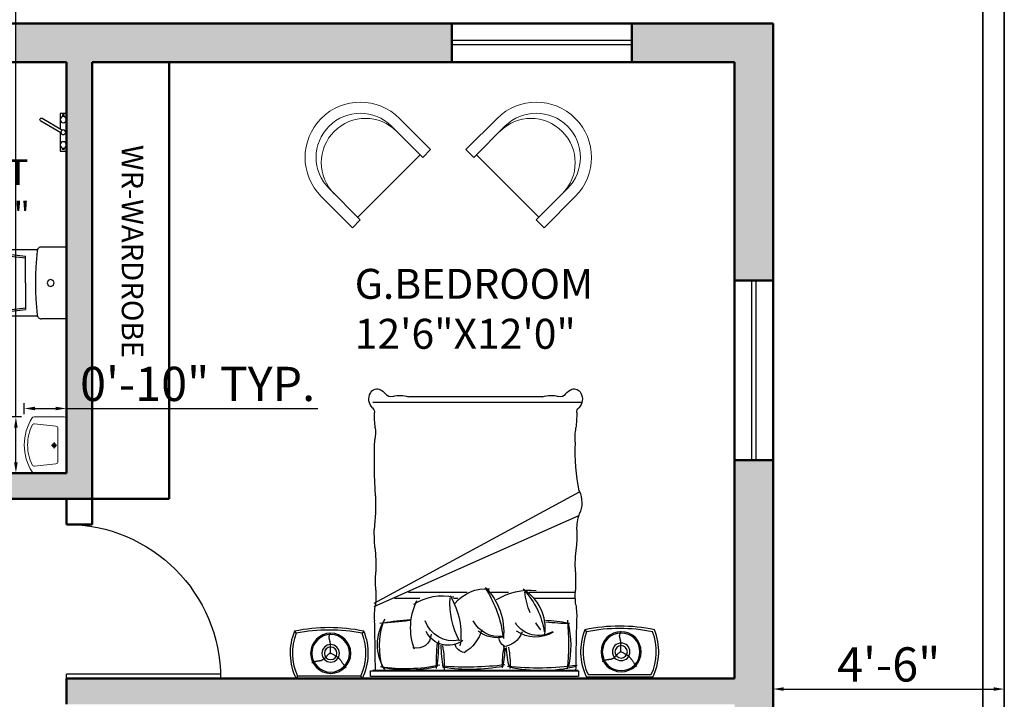
# Model space of a CAD drawing. Units: inches. Extents: x 3008 to 4088, y 1255 to 2137.
# Tile 29 of 30: x 3853 to 4083, y 1792 to 1951. Entities that reach past the tile are written whole.
import ezdxf

# ---------------------------------------------------------------- set-up
doc = ezdxf.new("R2010")
doc.units = ezdxf.units.IN
for name, color, linetype, lineweight in [('A-ANNO-DIMS', 2, 'Continuous', 18), ('A-ANNO-TEXT', 7, 'Continuous', 18), ('A-AREA-IDEN', 7, 'Continuous', 18), ('A-DOOR', 4, 'Continuous', 25), ('A-FLOR-FIXT', 8, 'Continuous', 18), ('A-FURN', 8, 'Continuous', 18), ('A-GLAZ', 4, 'Continuous', 25), ('A-WALL', 7, 'Continuous', 50), ('A-WALL-PATT', 8, 'Continuous', 13), ('C-PROP', 1, 'Continuous', 35)]:
    doc.layers.add(name, color=color, linetype=linetype, lineweight=lineweight)
doc.layers.add('SANTEH', color=7, linetype='Continuous')
doc.layers.add('TEFRİŞ', color=11, linetype='Continuous')
doc.styles.get("Standard").update_dxf_attribs({"font": 'arial.ttf'})
doc.dimstyles.new('ISO-25', dxfattribs={"dimtxt": 8, "dimasz": 2.5, "dimexe": 1.25, "dimexo": 0.625, "dimtad": 1, "dimdec": 1, "dimlunit": 3, "dimtxsty": 'Standard', "dimcen": 2.5, "dimadec": 0, "dimazin": 0, "dimtfac": 1, "dimtdec": 1, "dimtmove": 0, "dimatfit": 3, "dimfxl": 1, "dimarcsym": 0})

# ---------------------------------------------------------------- blocks, each defined once
blk = doc.blocks.new('*D34')
at = {"layer": 'A-ANNO-DIMS', "color": 0, "lineweight": -2, "transparency": 16777216}
for p, q in [((4028.94, 1793.63), (4028.94, 1793.01)), ((4031.44, 1794.26), (4080.44, 1794.26)), ((4082.94, 1793.63), (4082.94, 1793.01))]:
    blk.add_line(p, q, dxfattribs=at)
at = {"layer": 'A-ANNO-DIMS', "color": 0, "transparency": 16777216}
for points in [[(4031.44, 1794.68), (4031.44, 1793.84), (4028.94, 1794.26)], [(4080.44, 1794.68), (4080.44, 1793.84), (4082.94, 1794.26)]]:
    blk.add_solid(points, dxfattribs=at)
at = {"layer": 'Defpoints', "color": 0, "transparency": 16777216}
for p in [(4028.94, 1794.26), (4082.94, 1794.26), (4082.94, 1794.26)]:
    blk.add_point(p, dxfattribs=at)
at = {"layer": 'A-ANNO-DIMS', "color": 0, "transparency": 16777216, "insert": (4055.94, 1798.97), "char_height": 8, "attachment_point": 5}
blk.add_mtext('4\'-6"', dxfattribs=at)
blk = doc.blocks.new('WC 2 Symb_109')
at = {"layer": 'SANTEH'}
for p, q in [((0, 0), (0, 380)), ((0, 380), (132.4, 380)), ((153.6, 364.9), (506.8, 364.9)), ((506.3, 364.9), (215.7, 330.9)), ((506.3, 356), (215.7, 322)), ((215.7, 190), (215.7, 330.9)), ((215.7, 190), (215.7, 49.1)), ((506.3, 24), (215.7, 58)), ((153.8, 15.1), (506.8, 15.1)), ((506.3, 15.1), (215.7, 49.1)), ((0, 0), (132.4, 0))]:
    blk.add_line(p, q, dxfattribs=at)
for points in [[(154.6, 360.1), (153.9, 364.1), (152.3, 367.9), (150.2, 371.3), (147.4, 374.3), (144.1, 376.7), (140.5, 378.5), (136.5, 379.6), (132.4, 380)], [(506.8, 15.1), (569.2, 28.4), (622.2, 66.3), (657.6, 123.1), (670, 190), (657.6, 256.9), (622.2, 313.7), (569.2, 351.6), (506.8, 364.9)], [(154.6, 19.7), (158.6, 62.1), (161.4, 104.7), (163.1, 147.3), (163.7, 189.9), (163.1, 232.5), (161.4, 275.1), (158.6, 317.7), (154.6, 360.1)], [(506.3, 24), (565.5, 36.6), (615.7, 72.6), (649.2, 126.5), (661, 190), (649.2, 253.5), (615.7, 307.4), (565.5, 343.4), (506.3, 356)], [(132.4, 0), (136.5, 0.4), (140.4, 1.5), (144.1, 3.2), (147.3, 5.6), (150.1, 8.6), (152.3, 12), (153.8, 15.7), (154.6, 19.7)]]:
    blk.add_lwpolyline(points, dxfattribs=at)
blk.add_lwpolyline([(83.6, 208.5), (70.4, 203.1), (64.9, 190), (70.4, 176.9), (83.6, 171.5), (96.8, 176.9), (102.2, 190), (96.8, 203.1)], close=True, dxfattribs=at)
blk = doc.blocks.new('Faucet - kit sink top')
at = {"layer": 'SANTEH'}
for p, q in [((-5.5, -0.75), (-5.5, -1.25)), ((-4.94278, -0.75), (-5.5, -0.75)), ((-5.5, -1.25), (-4.94278, -1.25)), ((-0.14775, -1.7441), (3.56698, -8.1782)), ((4.43301, -7.6782), (0.71828, -1.2441)), ((4.94278, -0.75), (5.5, -0.75)), ((5.5, -1.25), (4.94278, -1.25)), ((5.5, -0.75), (5.5, -1.25))]:
    blk.add_line(p, q, dxfattribs=at)
blk.add_lwpolyline([(-0.00587, -2), (-6, -2), (-6, 0), (6, 0), (6, -2), (1.15195, -2)], dxfattribs=at)
for centre, radius in [((-4, -1), 1), ((4, -1), 1), ((0, -1), 0.75)]:
    blk.add_circle(centre, radius, dxfattribs=at)
blk.add_arc((4, -7.9282), 0.5, 210, 30, dxfattribs=at)
blk = doc.blocks.new('A$C2EBB240D')
for p, q in [((0, 355.8), (0, 86.6)), ((480, 375.8), (20, 375.8)), ((500, 355.8), (500, 86.6)), ((60.8, 89.8), (82.3, 282.2)), ((250, 300), (102.1, 300)), ((250, 300), (397.9, 300)), ((439.2, 89.8), (417.7, 282.2))]:
    blk.add_line(p, q)
for points in [[(275.2, 266.4), (219.4, 266.4)], [(247.3, 238.5), (247.3, 288.9)]]:
    blk.add_lwpolyline(points)
for centre, radius, start, end in [((20, 355.8), 20, 90, 180), ((480, 355.8), 20, 0, 90), ((102.1, 280), 20, 90, 173.64284), ((247.3, 266.4), 16.7, 90, 270), ((247.3, 266.4), 10, 90, 270), ((247.3, 266.4), 16.7, 270, 90), ((247.3, 266.4), 10, 270, 90), ((397.9, 280), 20, 6.35716, 90), ((80.7, 87.6), 20, 173.64284, 244.97956), ((419.3, 87.6), 20, 295.02044, 6.35716), ((20, 86.6), 20, 180, 237.68921), ((250, 450.3), 450.3, 237.68921, 270), ((250, 450.3), 420.3, 244.97956, 270), ((250, 450.3), 450.3, 270, 302.31079), ((250, 450.3), 420.3, 270, 295.02044), ((480, 86.6), 20, 302.31079, 0)]:
    blk.add_arc(centre, radius, start, end)
blk = doc.blocks.new('D1')
for p, q in [((1805.96, 1500.36), (1805.96, 1464.36)), ((1806.96, 1500.36), (1806.96, 1464.36)), ((1805.96, 1464.36), (1806.96, 1464.36))]:
    blk.add_line(p, q)
blk.add_arc((1805.96, 1464.36), 36, 0, 90)
blk = doc.blocks.new('12PSTG07')
at = {"color": 0, "linetype": 'ByBlock'}
for p, q in [((0, 15), (-12, 15)), ((0, 12), (0, 15)), ((-12, 12), (0, 12)), ((-1, -12), (-1, 12)), ((-12, -12), (0, -12)), ((0, -12), (0, -15)), ((0, -15), (-12, -15))]:
    blk.add_line(p, q, dxfattribs=at)
for centre, radius in [((-12, 0), 15), ((-12, 0), 12), ((-10, 0), 12)]:
    blk.add_arc(centre, radius, 90, 270, dxfattribs=at)
blk = doc.blocks.new('BED')
at = {"layer": 'TEFRİŞ'}
for p, q in [((2114.88, 1835.66), (2129.12, 1835.66)), ((2115.2, 1835.15), (2128.8, 1835.15)), ((2130.81, 1834.34), (2130.81, 1835.55)), ((2175.56, 1834.34), (2130.81, 1834.34)), ((2130.91, 1835.55), (2175.56, 1835.55)), ((2175, 1834.19), (2130.91, 1834.19)), ((2175.56, 1835.55), (2175.56, 1834.34)), ((2177.29, 1835.98), (2177.61, 1835.47)), ((2177.29, 1835.98), (2191.52, 1835.98)), ((2177.61, 1835.47), (2191.2, 1835.47)), ((2191.2, 1835.47), (2191.52, 1835.98)), ((2118.49, 1833.2), (2118.34, 1833.38)), ((2118.49, 1833.2), (2118.34, 1833.38)), ((2118.63, 1833.03), (2118.49, 1833.2)), ((2118.63, 1833.03), (2118.49, 1833.2)), ((2118.75, 1832.88), (2118.63, 1833.03)), ((2118.75, 1832.88), (2118.63, 1833.03)), ((2118.86, 1832.74), (2118.75, 1832.88)), ((2118.86, 1832.74), (2118.75, 1832.88)), ((2118.95, 1832.61), (2118.86, 1832.74)), ((2118.95, 1832.61), (2118.86, 1832.74)), ((2119.04, 1832.48), (2118.95, 1832.61)), ((2119.04, 1832.48), (2118.95, 1832.61)), ((2119.12, 1832.37), (2119.04, 1832.48)), ((2119.12, 1832.37), (2119.04, 1832.48)), ((2119.19, 1832.26), (2119.12, 1832.37)), ((2119.19, 1832.26), (2119.12, 1832.37)), ((2119.26, 1832.16), (2119.19, 1832.26)), ((2119.26, 1832.16), (2119.19, 1832.26)), ((2119.32, 1832.06), (2119.26, 1832.16)), ((2119.32, 1832.06), (2119.26, 1832.16)), ((2119.39, 1831.97), (2119.32, 1832.06)), ((2119.39, 1831.97), (2119.32, 1832.06)), ((2124.79, 1831.99), (2124.87, 1832.01)), ((2124.79, 1831.99), (2124.87, 1832.01)), ((2124.87, 1832.01), (2124.96, 1832.03)), ((2124.87, 1832.01), (2124.96, 1832.03)), ((2124.96, 1832.03), (2125.05, 1832.05)), ((2124.96, 1832.03), (2125.05, 1832.05)), ((2125.05, 1832.05), (2125.14, 1832.08)), ((2125.05, 1832.05), (2125.14, 1832.08)), ((2125.14, 1832.08), (2125.23, 1832.11)), ((2125.14, 1832.08), (2125.23, 1832.11)), ((2125.23, 1832.11), (2125.33, 1832.14)), ((2125.23, 1832.11), (2125.33, 1832.14)), ((2125.33, 1832.14), (2125.42, 1832.17)), ((2125.33, 1832.14), (2125.42, 1832.17)), ((2125.42, 1832.17), (2125.52, 1832.21)), ((2125.42, 1832.17), (2125.52, 1832.21)), ((2125.52, 1832.21), (2125.6, 1832.25)), ((2125.52, 1832.21), (2125.6, 1832.25)), ((2125.6, 1832.25), (2125.68, 1832.3)), ((2125.6, 1832.25), (2125.68, 1832.3)), ((2125.68, 1832.3), (2125.75, 1832.35)), ((2125.68, 1832.3), (2125.75, 1832.35)), ((2180.9, 1833.52), (2180.75, 1833.7)), ((2180.9, 1833.52), (2180.75, 1833.7)), ((2181.04, 1833.35), (2180.9, 1833.52)), ((2181.04, 1833.35), (2180.9, 1833.52)), ((2181.16, 1833.2), (2181.04, 1833.35)), ((2181.16, 1833.2), (2181.04, 1833.35)), ((2181.26, 1833.06), (2181.16, 1833.2)), ((2181.26, 1833.06), (2181.16, 1833.2)), ((2181.36, 1832.93), (2181.26, 1833.06)), ((2181.36, 1832.93), (2181.26, 1833.06)), ((2181.44, 1832.8), (2181.36, 1832.93)), ((2181.44, 1832.8), (2181.36, 1832.93)), ((2181.52, 1832.69), (2181.44, 1832.8)), ((2181.52, 1832.69), (2181.44, 1832.8)), ((2181.59, 1832.58), (2181.52, 1832.69)), ((2181.59, 1832.58), (2181.52, 1832.69)), ((2181.66, 1832.48), (2181.59, 1832.58)), ((2181.66, 1832.48), (2181.59, 1832.58)), ((2181.73, 1832.38), (2181.66, 1832.48)), ((2181.73, 1832.38), (2181.66, 1832.48)), ((2181.79, 1832.29), (2181.73, 1832.38)), ((2181.79, 1832.29), (2181.73, 1832.38)), ((2181.85, 1832.21), (2181.79, 1832.29)), ((2181.85, 1832.21), (2181.79, 1832.29)), ((2181.92, 1832.13), (2181.85, 1832.21)), ((2181.92, 1832.13), (2181.85, 1832.21)), ((2181.97, 1832.05), (2181.92, 1832.13)), ((2181.97, 1832.05), (2181.92, 1832.13)), ((2182.03, 1831.97), (2181.97, 1832.05)), ((2182.03, 1831.97), (2181.97, 1832.05)), ((2185.82, 1831.99), (2185.89, 1832.03)), ((2185.82, 1831.99), (2185.89, 1832.03)), ((2185.89, 1832.03), (2185.96, 1832.06)), ((2185.89, 1832.03), (2185.96, 1832.06)), ((2185.96, 1832.06), (2186.03, 1832.09)), ((2185.96, 1832.06), (2186.03, 1832.09)), ((2186.03, 1832.09), (2186.1, 1832.12)), ((2186.03, 1832.09), (2186.1, 1832.12)), ((2186.1, 1832.12), (2186.17, 1832.14)), ((2186.1, 1832.12), (2186.17, 1832.14)), ((2186.17, 1832.14), (2186.24, 1832.16)), ((2186.17, 1832.14), (2186.24, 1832.16)), ((2186.24, 1832.16), (2186.32, 1832.18)), ((2186.24, 1832.16), (2186.32, 1832.18)), ((2186.32, 1832.18), (2186.39, 1832.19)), ((2186.32, 1832.18), (2186.39, 1832.19)), ((2186.39, 1832.19), (2186.46, 1832.21)), ((2186.39, 1832.19), (2186.46, 1832.21)), ((2186.46, 1832.21), (2186.53, 1832.22)), ((2186.46, 1832.21), (2186.53, 1832.22)), ((2186.53, 1832.22), (2186.61, 1832.23)), ((2186.53, 1832.22), (2186.61, 1832.23)), ((2186.61, 1832.23), (2186.68, 1832.23)), ((2186.61, 1832.23), (2186.68, 1832.23)), ((2186.68, 1832.23), (2186.75, 1832.24)), ((2186.68, 1832.23), (2186.75, 1832.24)), ((2186.75, 1832.24), (2186.82, 1832.25)), ((2186.75, 1832.24), (2186.82, 1832.25)), ((2186.82, 1832.25), (2186.9, 1832.26)), ((2186.82, 1832.25), (2186.9, 1832.26)), ((2186.9, 1832.26), (2186.97, 1832.27)), ((2186.9, 1832.26), (2186.97, 1832.27)), ((2186.97, 1832.27), (2187.04, 1832.28)), ((2186.97, 1832.27), (2187.04, 1832.28)), ((2187.04, 1832.28), (2187.12, 1832.3)), ((2187.04, 1832.28), (2187.12, 1832.3)), ((2187.12, 1832.3), (2187.2, 1832.31)), ((2187.12, 1832.3), (2187.2, 1832.31)), ((2187.2, 1832.31), (2187.28, 1832.33)), ((2187.2, 1832.31), (2187.28, 1832.33)), ((2187.28, 1832.33), (2187.36, 1832.35)), ((2187.28, 1832.33), (2187.36, 1832.35)), ((2187.36, 1832.35), (2187.45, 1832.37)), ((2187.36, 1832.35), (2187.45, 1832.37)), ((2187.45, 1832.37), (2187.54, 1832.4)), ((2187.45, 1832.37), (2187.54, 1832.4)), ((2187.54, 1832.4), (2187.64, 1832.43)), ((2187.54, 1832.4), (2187.64, 1832.43)), ((2187.64, 1832.43), (2187.74, 1832.46)), ((2187.64, 1832.43), (2187.74, 1832.46)), ((2187.74, 1832.46), (2187.83, 1832.49)), ((2187.74, 1832.46), (2187.83, 1832.49)), ((2187.83, 1832.49), (2187.92, 1832.53)), ((2187.83, 1832.49), (2187.92, 1832.53)), ((2187.92, 1832.53), (2188.01, 1832.57)), ((2187.92, 1832.53), (2188.01, 1832.57)), ((2188.01, 1832.57), (2188.09, 1832.62)), ((2188.01, 1832.57), (2188.09, 1832.62)), ((2188.09, 1832.62), (2188.15, 1832.67)), ((2188.09, 1832.62), (2188.15, 1832.67)), ((2119.45, 1831.89), (2119.39, 1831.97)), ((2119.45, 1831.89), (2119.39, 1831.97)), ((2119.51, 1831.81), (2119.45, 1831.89)), ((2119.51, 1831.81), (2119.45, 1831.89)), ((2119.57, 1831.73), (2119.51, 1831.81)), ((2119.57, 1831.73), (2119.51, 1831.81)), ((2119.63, 1831.65), (2119.57, 1831.73)), ((2119.63, 1831.65), (2119.57, 1831.73)), ((2119.69, 1831.58), (2119.63, 1831.65)), ((2119.69, 1831.58), (2119.63, 1831.65)), ((2119.75, 1831.51), (2119.69, 1831.58)), ((2119.75, 1831.51), (2119.69, 1831.58)), ((2119.81, 1831.44), (2119.75, 1831.51)), ((2119.81, 1831.44), (2119.75, 1831.51)), ((2119.87, 1831.38), (2119.81, 1831.44)), ((2119.87, 1831.38), (2119.81, 1831.44)), ((2119.93, 1831.31), (2119.87, 1831.38)), ((2119.93, 1831.31), (2119.87, 1831.38)), ((2119.99, 1831.25), (2119.93, 1831.31)), ((2119.99, 1831.25), (2119.93, 1831.31)), ((2120.05, 1831.2), (2119.99, 1831.25)), ((2120.05, 1831.2), (2119.99, 1831.25)), ((2120.12, 1831.14), (2120.05, 1831.2)), ((2120.12, 1831.14), (2120.05, 1831.2)), ((2120.18, 1831.09), (2120.12, 1831.14)), ((2120.18, 1831.09), (2120.12, 1831.14)), ((2120.25, 1831.04), (2120.18, 1831.09)), ((2120.25, 1831.04), (2120.18, 1831.09)), ((2120.32, 1830.99), (2120.25, 1831.04)), ((2120.32, 1830.99), (2120.25, 1831.04)), ((2120.39, 1830.94), (2120.32, 1830.99)), ((2120.39, 1830.94), (2120.32, 1830.99)), ((2120.47, 1830.9), (2120.39, 1830.94)), ((2120.47, 1830.9), (2120.39, 1830.94)), ((2120.54, 1830.85), (2120.47, 1830.9)), ((2120.54, 1830.85), (2120.47, 1830.9)), ((2120.62, 1830.8), (2120.54, 1830.85)), ((2120.62, 1830.8), (2120.54, 1830.85)), ((2120.7, 1830.75), (2120.62, 1830.8)), ((2120.7, 1830.75), (2120.62, 1830.8)), ((2120.79, 1830.7), (2120.7, 1830.75)), ((2120.79, 1830.7), (2120.7, 1830.75)), ((2120.88, 1830.65), (2120.79, 1830.7)), ((2120.88, 1830.65), (2120.79, 1830.7)), ((2120.98, 1830.59), (2120.88, 1830.65)), ((2120.98, 1830.59), (2120.88, 1830.65)), ((2121.09, 1830.52), (2120.98, 1830.59)), ((2121.09, 1830.52), (2120.98, 1830.59)), ((2121.21, 1830.45), (2121.09, 1830.52)), ((2121.21, 1830.45), (2121.09, 1830.52)), ((2121.34, 1830.38), (2121.21, 1830.45)), ((2121.34, 1830.38), (2121.21, 1830.45)), ((2121.49, 1830.29), (2121.34, 1830.38)), ((2121.49, 1830.29), (2121.34, 1830.38)), ((2121.66, 1830.21), (2121.49, 1830.29)), ((2121.66, 1830.21), (2121.49, 1830.29)), ((2121.66, 1830.18), (2121.87, 1830.29)), ((2121.66, 1830.18), (2121.87, 1830.29)), ((2121.85, 1830.11), (2121.66, 1830.21)), ((2121.85, 1830.11), (2121.66, 1830.21)), ((2121.74, 1829.99), (2121.73, 1829.83)), ((2121.74, 1829.99), (2121.73, 1829.83)), ((2121.76, 1830.38), (2121.74, 1830.17)), ((2121.76, 1830.38), (2121.74, 1830.17)), ((2121.74, 1830.17), (2121.74, 1829.99)), ((2121.74, 1830.17), (2121.74, 1829.99)), ((2121.87, 1830.29), (2122.04, 1830.4)), ((2121.87, 1830.29), (2122.04, 1830.4)), ((2122.04, 1830.4), (2122.2, 1830.51)), ((2122.04, 1830.4), (2122.2, 1830.51)), ((2122.2, 1830.51), (2122.33, 1830.61)), ((2122.2, 1830.51), (2122.33, 1830.61)), ((2122.33, 1830.61), (2122.45, 1830.72)), ((2122.33, 1830.61), (2122.45, 1830.72)), ((2122.45, 1830.72), (2122.55, 1830.82)), ((2122.45, 1830.72), (2122.55, 1830.82)), ((2122.55, 1830.82), (2122.64, 1830.91)), ((2122.55, 1830.82), (2122.64, 1830.91)), ((2122.64, 1830.91), (2122.72, 1831.01)), ((2122.64, 1830.91), (2122.72, 1831.01)), ((2122.72, 1831.01), (2122.8, 1831.09)), ((2122.72, 1831.01), (2122.8, 1831.09)), ((2122.8, 1831.09), (2122.87, 1831.18)), ((2122.8, 1831.09), (2122.87, 1831.18)), ((2122.87, 1831.18), (2122.94, 1831.26)), ((2122.87, 1831.18), (2122.94, 1831.26)), ((2122.94, 1831.26), (2123.01, 1831.33)), ((2122.94, 1831.26), (2123.01, 1831.33)), ((2123.01, 1831.33), (2123.08, 1831.4)), ((2123.01, 1831.33), (2123.08, 1831.4)), ((2123.08, 1831.4), (2123.14, 1831.46)), ((2123.08, 1831.4), (2123.14, 1831.46)), ((2123.14, 1831.46), (2123.21, 1831.52)), ((2123.14, 1831.46), (2123.21, 1831.52)), ((2123.21, 1831.52), (2123.27, 1831.58)), ((2123.21, 1831.52), (2123.27, 1831.58)), ((2123.27, 1831.58), (2123.34, 1831.63)), ((2123.27, 1831.58), (2123.34, 1831.63)), ((2123.34, 1831.63), (2123.41, 1831.67)), ((2123.34, 1831.63), (2123.41, 1831.67)), ((2123.41, 1831.67), (2123.48, 1831.71)), ((2123.41, 1831.67), (2123.48, 1831.71)), ((2123.48, 1831.71), (2123.55, 1831.74)), ((2123.48, 1831.71), (2123.55, 1831.74)), ((2123.55, 1831.74), (2123.62, 1831.77)), ((2123.55, 1831.74), (2123.62, 1831.77)), ((2123.62, 1831.77), (2123.69, 1831.8)), ((2123.62, 1831.77), (2123.69, 1831.8)), ((2123.69, 1831.8), (2123.77, 1831.82)), ((2123.69, 1831.8), (2123.77, 1831.82)), ((2123.77, 1831.82), (2123.84, 1831.84)), ((2123.77, 1831.82), (2123.84, 1831.84)), ((2123.84, 1831.84), (2123.91, 1831.86)), ((2123.84, 1831.84), (2123.91, 1831.86)), ((2123.91, 1831.86), (2123.98, 1831.87)), ((2123.91, 1831.86), (2123.98, 1831.87)), ((2123.98, 1831.87), (2124.06, 1831.89)), ((2123.98, 1831.87), (2124.06, 1831.89)), ((2124.06, 1831.89), (2124.13, 1831.9)), ((2124.06, 1831.89), (2124.13, 1831.9)), ((2124.13, 1831.9), (2124.2, 1831.91)), ((2124.13, 1831.9), (2124.2, 1831.91)), ((2124.2, 1831.91), (2124.27, 1831.91)), ((2124.2, 1831.91), (2124.27, 1831.91)), ((2124.27, 1831.91), (2124.35, 1831.92)), ((2124.27, 1831.91), (2124.35, 1831.92)), ((2124.35, 1831.92), (2124.42, 1831.93)), ((2124.35, 1831.92), (2124.42, 1831.93)), ((2124.42, 1831.93), (2124.49, 1831.94)), ((2124.42, 1831.93), (2124.49, 1831.94)), ((2124.49, 1831.94), (2124.56, 1831.95)), ((2124.49, 1831.94), (2124.56, 1831.95)), ((2124.56, 1831.95), (2124.64, 1831.96)), ((2124.56, 1831.95), (2124.64, 1831.96)), ((2124.64, 1831.96), (2124.71, 1831.98)), ((2124.64, 1831.96), (2124.71, 1831.98)), ((2124.71, 1831.98), (2124.79, 1831.99)), ((2124.71, 1831.98), (2124.79, 1831.99)), ((2182.09, 1831.9), (2182.03, 1831.97)), ((2182.09, 1831.9), (2182.03, 1831.97)), ((2182.15, 1831.83), (2182.09, 1831.9)), ((2182.15, 1831.83), (2182.09, 1831.9)), ((2182.21, 1831.76), (2182.15, 1831.83)), ((2182.21, 1831.76), (2182.15, 1831.83)), ((2182.27, 1831.7), (2182.21, 1831.76)), ((2182.27, 1831.7), (2182.21, 1831.76)), ((2182.33, 1831.63), (2182.27, 1831.7)), ((2182.33, 1831.63), (2182.27, 1831.7)), ((2182.4, 1831.57), (2182.33, 1831.63)), ((2182.4, 1831.57), (2182.33, 1831.63)), ((2182.46, 1831.52), (2182.4, 1831.57)), ((2182.46, 1831.52), (2182.4, 1831.57)), ((2182.52, 1831.46), (2182.46, 1831.52)), ((2182.52, 1831.46), (2182.46, 1831.52)), ((2182.59, 1831.41), (2182.52, 1831.46)), ((2182.59, 1831.41), (2182.52, 1831.46)), ((2182.66, 1831.36), (2182.59, 1831.41)), ((2182.66, 1831.36), (2182.59, 1831.41)), ((2182.73, 1831.31), (2182.66, 1831.36)), ((2182.73, 1831.31), (2182.66, 1831.36)), ((2182.8, 1831.26), (2182.73, 1831.31)), ((2182.8, 1831.26), (2182.73, 1831.31)), ((2182.87, 1831.22), (2182.8, 1831.26)), ((2182.87, 1831.22), (2182.8, 1831.26)), ((2182.95, 1831.17), (2182.87, 1831.22)), ((2182.95, 1831.17), (2182.87, 1831.22)), ((2183.03, 1831.12), (2182.95, 1831.17)), ((2183.03, 1831.12), (2182.95, 1831.17)), ((2183.11, 1831.07), (2183.03, 1831.12)), ((2183.11, 1831.07), (2183.03, 1831.12)), ((2183.2, 1831.02), (2183.11, 1831.07)), ((2183.2, 1831.02), (2183.11, 1831.07)), ((2183.29, 1830.97), (2183.2, 1831.02)), ((2183.29, 1830.97), (2183.2, 1831.02)), ((2183.39, 1830.91), (2183.29, 1830.97)), ((2183.39, 1830.91), (2183.29, 1830.97)), ((2183.49, 1830.84), (2183.39, 1830.91)), ((2183.49, 1830.84), (2183.39, 1830.91)), ((2183.61, 1830.77), (2183.49, 1830.84)), ((2183.61, 1830.77), (2183.49, 1830.84)), ((2183.75, 1830.7), (2183.61, 1830.77)), ((2183.75, 1830.7), (2183.61, 1830.77)), ((2183.9, 1830.61), (2183.75, 1830.7)), ((2183.9, 1830.61), (2183.75, 1830.7)), ((2184.06, 1830.53), (2183.9, 1830.61)), ((2184.06, 1830.53), (2183.9, 1830.61)), ((2184.25, 1830.43), (2184.06, 1830.53)), ((2184.25, 1830.43), (2184.06, 1830.53)), ((2184.07, 1830.5), (2184.27, 1830.61)), ((2184.07, 1830.5), (2184.27, 1830.61)), ((2184.15, 1830.49), (2184.14, 1830.31)), ((2184.15, 1830.49), (2184.14, 1830.31)), ((2184.14, 1830.31), (2184.14, 1830.15)), ((2184.14, 1830.31), (2184.14, 1830.15)), ((2184.14, 1830.15), (2184.14, 1830.01)), ((2184.14, 1830.15), (2184.14, 1830.01)), ((2184.14, 1830.01), (2184.14, 1829.89)), ((2184.14, 1830.01), (2184.14, 1829.89)), ((2184.14, 1829.89), (2184.14, 1829.77)), ((2184.14, 1829.89), (2184.14, 1829.77)), ((2184.17, 1830.7), (2184.15, 1830.49)), ((2184.17, 1830.7), (2184.15, 1830.49)), ((2184.27, 1830.61), (2184.45, 1830.72)), ((2184.27, 1830.61), (2184.45, 1830.72)), ((2184.45, 1830.72), (2184.6, 1830.83)), ((2184.45, 1830.72), (2184.6, 1830.83)), ((2184.6, 1830.83), (2184.74, 1830.93)), ((2184.6, 1830.83), (2184.74, 1830.93)), ((2184.74, 1830.93), (2184.85, 1831.04)), ((2184.74, 1830.93), (2184.85, 1831.04)), ((2184.85, 1831.04), (2184.95, 1831.14)), ((2184.85, 1831.04), (2184.95, 1831.14)), ((2184.95, 1831.14), (2185.05, 1831.23)), ((2184.95, 1831.14), (2185.05, 1831.23)), ((2185.05, 1831.23), (2185.13, 1831.33)), ((2185.05, 1831.23), (2185.13, 1831.33)), ((2185.13, 1831.33), (2185.21, 1831.41)), ((2185.13, 1831.33), (2185.21, 1831.41)), ((2185.21, 1831.41), (2185.28, 1831.5)), ((2185.21, 1831.41), (2185.28, 1831.5)), ((2185.28, 1831.5), (2185.35, 1831.58)), ((2185.28, 1831.5), (2185.35, 1831.58)), ((2185.35, 1831.58), (2185.42, 1831.65)), ((2185.35, 1831.58), (2185.42, 1831.65)), ((2185.42, 1831.65), (2185.48, 1831.72)), ((2185.42, 1831.65), (2185.48, 1831.72)), ((2185.48, 1831.72), (2185.55, 1831.78)), ((2185.48, 1831.72), (2185.55, 1831.78)), ((2185.55, 1831.78), (2185.61, 1831.84)), ((2185.55, 1831.78), (2185.61, 1831.84)), ((2185.61, 1831.84), (2185.68, 1831.9)), ((2185.61, 1831.84), (2185.68, 1831.9)), ((2185.68, 1831.9), (2185.75, 1831.95)), ((2185.68, 1831.9), (2185.75, 1831.95)), ((2185.75, 1831.95), (2185.82, 1831.99)), ((2185.75, 1831.95), (2185.82, 1831.99)), ((2121.73, 1829.83), (2121.73, 1829.69)), ((2121.73, 1829.83), (2121.73, 1829.69)), ((2121.73, 1829.69), (2121.73, 1829.57)), ((2121.73, 1829.69), (2121.73, 1829.57)), ((2121.73, 1829.57), (2121.73, 1829.45)), ((2121.73, 1829.57), (2121.73, 1829.45)), ((2121.73, 1829.45), (2121.74, 1829.35)), ((2121.73, 1829.45), (2121.74, 1829.35)), ((2121.74, 1828.89), (2121.73, 1828.8)), ((2121.74, 1828.89), (2121.73, 1828.8)), ((2121.73, 1828.8), (2121.73, 1828.72)), ((2121.73, 1828.8), (2121.73, 1828.72)), ((2121.73, 1828.72), (2121.73, 1828.64)), ((2121.73, 1828.72), (2121.73, 1828.64)), ((2121.73, 1828.64), (2121.73, 1828.56)), ((2121.73, 1828.64), (2121.73, 1828.56)), ((2121.73, 1828.56), (2121.73, 1828.48)), ((2121.73, 1828.56), (2121.73, 1828.48)), ((2121.73, 1828.48), (2121.73, 1828.4)), ((2121.73, 1828.48), (2121.73, 1828.4)), ((2121.73, 1828.4), (2121.73, 1828.33)), ((2121.73, 1828.4), (2121.73, 1828.33)), ((2121.73, 1828.33), (2121.74, 1828.25)), ((2121.73, 1828.33), (2121.74, 1828.25)), ((2121.74, 1829.35), (2121.74, 1829.25)), ((2121.74, 1829.35), (2121.74, 1829.25)), ((2121.74, 1829.25), (2121.74, 1829.16)), ((2121.74, 1829.25), (2121.74, 1829.16)), ((2121.74, 1829.16), (2121.74, 1829.06)), ((2121.74, 1829.16), (2121.74, 1829.06)), ((2121.74, 1829.06), (2121.74, 1828.97)), ((2121.74, 1829.06), (2121.74, 1828.97)), ((2121.74, 1828.97), (2121.74, 1828.89)), ((2121.74, 1828.97), (2121.74, 1828.89)), ((2121.74, 1828.25), (2121.75, 1828.18)), ((2121.74, 1828.25), (2121.75, 1828.18)), ((2121.75, 1828.18), (2121.75, 1828.1)), ((2121.75, 1828.18), (2121.75, 1828.1)), ((2121.75, 1828.1), (2121.76, 1828.03)), ((2121.75, 1828.1), (2121.76, 1828.03)), ((2121.76, 1828.03), (2121.78, 1827.95)), ((2121.76, 1828.03), (2121.78, 1827.95)), ((2121.78, 1827.95), (2121.79, 1827.88)), ((2121.78, 1827.95), (2121.79, 1827.88)), ((2121.79, 1827.88), (2121.8, 1827.8)), ((2121.79, 1827.88), (2121.8, 1827.8)), ((2121.8, 1827.8), (2121.82, 1827.72)), ((2121.8, 1827.8), (2121.82, 1827.72)), ((2184.14, 1829.04), (2184.13, 1828.96)), ((2184.14, 1829.04), (2184.13, 1828.96)), ((2184.13, 1828.96), (2184.13, 1828.88)), ((2184.13, 1828.96), (2184.13, 1828.88)), ((2184.13, 1828.88), (2184.13, 1828.8)), ((2184.13, 1828.88), (2184.13, 1828.8)), ((2184.13, 1828.8), (2184.14, 1828.72)), ((2184.13, 1828.8), (2184.14, 1828.72)), ((2184.14, 1829.77), (2184.14, 1829.67)), ((2184.14, 1829.77), (2184.14, 1829.67)), ((2184.14, 1829.67), (2184.15, 1829.57)), ((2184.14, 1829.67), (2184.15, 1829.57)), ((2184.15, 1829.38), (2184.14, 1829.29)), ((2184.15, 1829.38), (2184.14, 1829.29)), ((2184.14, 1829.29), (2184.14, 1829.21)), ((2184.14, 1829.29), (2184.14, 1829.21)), ((2184.14, 1829.21), (2184.14, 1829.12)), ((2184.14, 1829.21), (2184.14, 1829.12)), ((2184.14, 1829.12), (2184.14, 1829.04)), ((2184.14, 1829.12), (2184.14, 1829.04)), ((2184.14, 1828.72), (2184.14, 1828.65)), ((2184.14, 1828.72), (2184.14, 1828.65)), ((2184.14, 1828.65), (2184.15, 1828.57)), ((2184.14, 1828.65), (2184.15, 1828.57)), ((2184.15, 1829.57), (2184.15, 1829.48)), ((2184.15, 1829.57), (2184.15, 1829.48)), ((2184.15, 1829.48), (2184.15, 1829.38)), ((2184.15, 1829.48), (2184.15, 1829.38)), ((2184.15, 1828.57), (2184.15, 1828.5)), ((2184.15, 1828.57), (2184.15, 1828.5)), ((2184.15, 1828.5), (2184.16, 1828.42)), ((2184.15, 1828.5), (2184.16, 1828.42)), ((2184.16, 1828.42), (2184.17, 1828.35)), ((2184.16, 1828.42), (2184.17, 1828.35)), ((2184.17, 1828.35), (2184.18, 1828.27)), ((2184.17, 1828.35), (2184.18, 1828.27)), ((2184.18, 1828.27), (2184.19, 1828.2)), ((2184.18, 1828.27), (2184.19, 1828.2)), ((2184.19, 1828.2), (2184.21, 1828.12)), ((2184.19, 1828.2), (2184.21, 1828.12)), ((2184.21, 1828.12), (2184.22, 1828.04)), ((2184.21, 1828.12), (2184.22, 1828.04)), ((2184.22, 1828.04), (2184.24, 1827.97)), ((2184.22, 1828.04), (2184.24, 1827.97)), ((2184.24, 1827.97), (2184.26, 1827.89)), ((2184.24, 1827.97), (2184.26, 1827.89)), ((2184.26, 1827.89), (2184.28, 1827.81)), ((2184.26, 1827.89), (2184.28, 1827.81)), ((2184.28, 1827.81), (2184.3, 1827.73)), ((2184.28, 1827.81), (2184.3, 1827.73)), ((2121.78, 1825.93), (2121.74, 1825.8)), ((2121.78, 1825.93), (2121.74, 1825.8)), ((2121.83, 1826.06), (2121.78, 1825.93)), ((2121.83, 1826.06), (2121.78, 1825.93)), ((2121.82, 1827.72), (2121.84, 1827.65)), ((2121.82, 1827.72), (2121.84, 1827.65)), ((2121.87, 1826.19), (2121.83, 1826.06)), ((2121.87, 1826.19), (2121.83, 1826.06)), ((2121.84, 1827.65), (2121.85, 1827.57)), ((2121.84, 1827.65), (2121.85, 1827.57)), ((2121.85, 1827.57), (2121.87, 1827.49)), ((2121.85, 1827.57), (2121.87, 1827.49)), ((2121.87, 1827.49), (2121.89, 1827.41)), ((2121.87, 1827.49), (2121.89, 1827.41)), ((2121.91, 1826.31), (2121.87, 1826.19)), ((2121.91, 1826.31), (2121.87, 1826.19)), ((2121.89, 1827.41), (2121.91, 1827.33)), ((2121.89, 1827.41), (2121.91, 1827.33)), ((2121.91, 1827.33), (2121.93, 1827.26)), ((2121.91, 1827.33), (2121.93, 1827.26)), ((2121.95, 1826.42), (2121.91, 1826.31)), ((2121.95, 1826.42), (2121.91, 1826.31)), ((2121.93, 1827.26), (2121.95, 1827.18)), ((2121.93, 1827.26), (2121.95, 1827.18)), ((2121.95, 1827.18), (2121.97, 1827.09)), ((2121.95, 1827.18), (2121.97, 1827.09)), ((2121.97, 1826.54), (2121.95, 1826.42)), ((2121.97, 1826.54), (2121.95, 1826.42)), ((2121.97, 1827.09), (2121.99, 1827.01)), ((2121.97, 1827.09), (2121.99, 1827.01)), ((2121.99, 1826.64), (2121.97, 1826.54)), ((2121.99, 1826.64), (2121.97, 1826.54)), ((2121.99, 1827.01), (2122, 1826.93)), ((2121.99, 1827.01), (2122, 1826.93)), ((2122, 1826.74), (2121.99, 1826.64)), ((2122, 1826.74), (2121.99, 1826.64)), ((2122, 1826.93), (2122.01, 1826.84)), ((2122, 1826.93), (2122.01, 1826.84)), ((2122.01, 1826.84), (2122, 1826.74)), ((2122.01, 1826.84), (2122, 1826.74)), ((2129.46, 1825.49), (2129.09, 1825.93)), ((2176.94, 1825.81), (2177.31, 1826.25)), ((2184.19, 1826.25), (2184.14, 1826.12)), ((2184.19, 1826.25), (2184.14, 1826.12)), ((2184.23, 1826.38), (2184.19, 1826.25)), ((2184.23, 1826.38), (2184.19, 1826.25)), ((2184.28, 1826.51), (2184.23, 1826.38)), ((2184.28, 1826.51), (2184.23, 1826.38)), ((2184.32, 1826.63), (2184.28, 1826.51)), ((2184.32, 1826.63), (2184.28, 1826.51)), ((2184.3, 1827.73), (2184.32, 1827.65)), ((2184.3, 1827.73), (2184.32, 1827.65)), ((2184.32, 1827.65), (2184.34, 1827.58)), ((2184.32, 1827.65), (2184.34, 1827.58)), ((2184.35, 1826.74), (2184.32, 1826.63)), ((2184.35, 1826.74), (2184.32, 1826.63)), ((2184.34, 1827.58), (2184.36, 1827.5)), ((2184.34, 1827.58), (2184.36, 1827.5)), ((2184.38, 1826.86), (2184.35, 1826.74)), ((2184.38, 1826.86), (2184.35, 1826.74)), ((2184.36, 1827.5), (2184.38, 1827.41)), ((2184.36, 1827.5), (2184.38, 1827.41)), ((2184.38, 1827.41), (2184.4, 1827.33)), ((2184.38, 1827.41), (2184.4, 1827.33)), ((2184.4, 1826.96), (2184.38, 1826.86)), ((2184.4, 1826.96), (2184.38, 1826.86)), ((2184.4, 1827.33), (2184.41, 1827.25)), ((2184.4, 1827.33), (2184.41, 1827.25)), ((2184.41, 1827.06), (2184.4, 1826.96)), ((2184.41, 1827.06), (2184.4, 1826.96)), ((2184.41, 1827.25), (2184.41, 1827.16)), ((2184.41, 1827.25), (2184.41, 1827.16)), ((2184.41, 1827.16), (2184.41, 1827.06)), ((2184.41, 1827.16), (2184.41, 1827.06)), ((2191.87, 1825.81), (2191.5, 1826.25)), ((2174.77, 1819.77), (2130.6, 1795.83)), ((2174.77, 1820.53), (2130.76, 1800.91)), ((2140.43, 1818.69), (2131.53, 1818.69)), ((2141.43, 1817.4), (2131.53, 1817.4)), ((2149.62, 1817.4), (2145.88, 1817.4)), ((2167.36, 1817.4), (2154.77, 1817.4)), ((2157.71, 1818.69), (2156.77, 1818.69)), ((2170.41, 1818.69), (2164.92, 1818.69)), ((2175, 1776.57), (2130.11, 1776.57)), ((2138.52, 1775.41), (2167.39, 1775.41))]:
    blk.add_line(p, q, dxfattribs=at)
for centre, radius, start, end in [((2126, 1830.19), 12.39, 153.8162, 202.314), ((2126, 1830.19), 11.88, 155.3335, 201.0157), ((2118, 1830.19), 11.88, 338.9843, 24.6665), ((2118, 1830.19), 12.39, 337.686, 26.1838), ((2188.4, 1830.51), 12.39, 153.8162, 202.314), ((2188.4, 1830.51), 11.88, 155.3335, 201.0157), ((2180.41, 1830.51), 11.88, 338.9843, 24.6665), ((2180.41, 1830.51), 12.39, 337.686, 26.1838), ((2122, 1861.35), 36.12, 258.6773, 281.3227), ((2184.41, 1861.67), 36.63, 258.2443, 281.7557), ((2184.41, 1861.67), 36.12, 258.6773, 281.3227), ((2122, 1861.35), 36.63, 258.2443, 281.7557)]:
    blk.add_arc(centre, radius, start, end, dxfattribs=at)
at = {"layer": 'TEFRİŞ', "extrusion": (0, 0, -1)}
for centre, major_axis, ratio, start_param, end_param in [((2121.68, 1830.24), (-3.05, -3.05), 1, 3.926991, 10.210176), ((2121.68, 1830.24), (2.86, -2.86), 1, 5.497787, 11.780972), ((2121.68, 1830.24), (2.86, -2.86), 1, 5.497787, 11.780972), ((2206.14, 1830.73), (-52.86, -52.86), 1, 0.767743, 0.83177), ((2138.85, 1803.05), (-22.1, 22.1), 1, 0.544604, 1.006234), ((2154.12, 1796.61), (-26.46, 26.46), 1, 0.596409, 0.940188), ((2168.35, 1789.27), (-1.33, 44.62), 0.875277, -0.163954, 0.163954), ((2167.6, 1797.72), (-0.51, 36.47), 0.865194, -0.185965, 0.185965), ((2184.09, 1830.56), (-3.05, -3.05), 1, 3.926991, 10.210176), ((2184.09, 1830.56), (2.86, -2.86), 1, 5.497787, 11.780972), ((2184.09, 1830.56), (2.86, -2.86), 1, 5.497787, 11.780972), ((2121.68, 1830.24), (1.33, -1.33), 1, 5.497787, 11.780972), ((2121.68, 1830.24), (1.33, -1.33), 1, 5.497787, 11.780972), ((2139.43, 1773.84), (-42.35, 42.35), 1, 0.646251, 0.896949), ((2154.7, 1828.89), (-15.68, 15.68), 1, -1.00675, -0.580436), ((2181.61, 1828.44), (-34.39, 34.39), 1, -0.888486, -0.672463), ((2164.51, 1832.79), (-13.41, 13.41), 1, -0.974476, -0.730892), ((2127.6, 1828.81), (-13.23, 13.23), 1, 2.100388, 2.328052), ((2155, 1761.9), (-50.65, -50.65), 1, 2.239512, 2.426533), ((2172.01, 1828.66), (-17.93, 17.93), 1, -0.753394, -0.598744), ((2128.44, 1832.96), (-13.26, -13.26), 1, 3.889049, 4.127298), ((2183.72, 1833.22), (-17, 17), 1, -0.967105, -0.749712), ((2134, 1828.8), (-18.62, 18.62), 1, 2.173461, 2.355043), ((2199.2, 1828.45), (-27.06, -27.06), 1, 0.770625, 0.917228), ((2087.32, 1833.96), (-52.37, 52.37), 1, 2.358049, 2.431787), ((2164.15, 1828.7), (-6.99, 6.99), 1, 1.789136, 2.946702), ((2156.76, 1828.98), (-11.9, -11.9), 1, 3.646453, 4.226155), ((2099.77, 1830.73), (-52.86, 52.86), 1, 2.311571, 2.373849), ((2184.09, 1830.56), (1.33, -1.33), 1, 5.497787, 11.780972), ((2184.09, 1830.56), (1.33, -1.33), 1, 5.497787, 11.780972), ((2184.09, 1830.56), (0.952, -0.952), 1, 5.497787, 11.780972), ((2184.09, 1830.56), (0.952, -0.952), 1, 5.497787, 11.780972), ((2121.68, 1830.24), (0.952, -0.952), 1, 5.497787, 11.780972), ((2121.68, 1830.24), (0.952, -0.952), 1, 5.497787, 11.780972), ((2159.55, 1823.33), (-5.81, 5.81), 1, -0.516587, 0.256776), ((2154.84, 1827.75), (-1.93, 1.93), 1, 0.997904, 1.977819), ((2675.38, 1815.09), (-384.79, -384.79), 1, 0.80103, 0.811711), ((2147.44, 1824.41), (-3.36, -3.36), 1, 1.11934, 2.270556), ((2145.66, 1827.01), (-1.62, 1.62), 1, 1.310976, 2.284591), ((2172, 1826.44), (-11.23, 11.23), 1, -1.332486, -0.624868), ((2158.82, 1823.55), (-3.74, -3.74), 1, 1.730792, 3.47045), ((2141.71, 1819.83), (-11.86, 11.86), 1, 1.850844, 2.42862), ((2157.83, 1821.53), (-4.47, 4.47), 1, 0.576679, 2.021689), ((2166.67, 1824.96), (-2.93, 3.91), 0.760601, -0.723751, 0.723751), ((2153.88, 1825.05), (-9.22, 9.22), 1, 1.994956, 2.818753), ((1630.53, 1815.09), (-384.79, 384.79), 1, 2.329881, 2.340562), ((2140.05, 1819.86), (-5.1, 5.1), 1, 0.238357, 1.390139), ((2139.42, 1820.79), (-4.21, -4.21), 1, 1.82161, 3.349145), ((2148.15, 1825.25), (-7.14, -7.14), 1, 6.061986, 7.190757), ((2154.93, 1828.48), (-11.96, 11.96), 1, -1.530302, -0.934407), ((2160.6, 1825.98), (-9.68, -9.68), 1, 0.009196, 0.886853), ((2148.35, 1820.65), (-4.63, -4.63), 1, 2.117602, 3.020837), ((2147.86, 1820.64), (-4.48, 4.48), 1, 0.665914, 1.867503), ((2170.68, 1829.67), (-16.79, 16.79), 1, -1.354718, -0.902276), ((2146.08, 1822.57), (-10.5, 10.5), 1, -0.951783, -0.716225), ((2132.43, 1774.09), (-35.41, -35.41), 1, 2.362911, 2.464592), ((2140.17, 1862.96), (-27.99, 27.99), 1, 3.983025, 4.107469), ((2127.37, 1815.76), (-10.68, 10.68), 1, 1.657204, 1.779381), ((2165.73, 1860.69), (-26.41, -26.41), 1, 5.306413, 5.463767), ((2199.62, 1529.47), (-209.2, 209.2), 1, 0.675361, 0.697001), ((2159.82, 1822.57), (-10.5, -10.5), 1, 3.857817, 4.093375), ((2127.37, 1815.76), (-10.68, 10.68), 1, 1.94252, 2.248924), ((2111.06, 1818.12), (-14.48, 14.48), 1, 2.258605, 2.412359), ((2150.79, 1825.18), (-6, 6), 1, 3.032122, 4.026148), ((2159.02, 1834.9), (-3.04, 16.53), 0.830169, 2.822117, 3.461068), ((2194.85, 1818.12), (-14.48, 14.48), 1, -0.841563, -0.687809), ((2141.33, 1830.48), (-9.55, -9.55), 1, 4.941413, 5.601673), ((2169.92, 1815.01), (-27.2, -27.2), 1, 0.734393, 0.836404), ((2135.98, 1815.01), (-27.2, -27.2), 1, 3.875985, 3.977996), ((2098.24, 1811.68), (-23.54, -23.54), 1, 3.885834, 4.043401), ((2207.66, 1811.68), (-23.54, -23.54), 1, 0.668988, 0.826555), ((2189.03, 1803.74), (-40.91, -40.91), 1, 0.789771, 0.855756), ((2116.87, 1803.74), (-40.91, 40.91), 1, 2.285836, 2.351822), ((2122.14, 1803.63), (-6.39, -6.39), 1, 3.886359, 4.265474), ((2222.76, 1798.77), (-34.16, -34.16), 1, 0.743488, 0.893627), ((2135.02, 1798.41), (-3.45, 3.45), 1, -0.831635, -0.314979), ((2135.48, 1798), (-3.77, -3.77), 1, 0.329385, 0.820948), ((2148.06, 1790.38), (-0.75, 67.37), 0.394952, 1.480524, 1.661068), ((2127.76, 1790.23), (-1, 12.37), 0.296708, 1.141067, 2.000525), ((2118.49, 1784.2), (-9.24, -9.24), 1, 3.839645, 4.088086), ((2182.27, 1782.99), (-5.52, -5.52), 1, 0.671703, 0.993321), ((2162.12, 1778.86), (-21.85, 21.85), 1, -0.78611, -0.680117), ((2143.78, 1778.86), (-21.85, 21.85), 1, 2.250913, 2.356906), ((2132.72, 1775.92), (-1.91, -1.91), 1, 0.284117, 1.557111), ((2129.83, 1778.8), (-0.986, 0.986), 1, 2.330985, 3.163296), ((2176.08, 1778.8), (-0.986, 0.986), 1, 4.690686, 5.522997), ((2173.18, 1775.92), (-1.91, -1.91), 1, 3.155278, 4.428271), ((2134.73, 1774.06), (-0.964, -0.964), 1, 1.381176, 2.701227), ((2136.75, 1781.14), (-4.24, 4.24), 1, 3.62713, 4.188813), ((2169.16, 1781.14), (-4.24, 4.24), 1, 3.665169, 4.226852), ((2171.17, 1774.06), (-0.964, -0.964), 1, 2.011162, 3.331212), ((2131.79, 1775.28), (-1.11, 1.11), 1, 3.629269, 5.067473), ((2130.83, 1777), (-2.49, -2.49), 1, 4.590984, 5.084038), ((2175.07, 1777), (-2.49, 2.49), 1, 4.34074, 4.833793), ((2174.12, 1775.28), (-1.11, 1.11), 1, 2.786508, 4.224712)]:
    blk.add_ellipse(centre, major_axis=major_axis, ratio=ratio, start_param=start_param, end_param=end_param, dxfattribs=at)
blk = doc.blocks.new('*D47')
at = {"layer": 'A-ANNO-DIMS', "color": 0, "lineweight": -2, "transparency": 16777216}
for p, q in [((3852.13, 1857.83), (3852.13, 1983.94)), ((3853.47, 1857.83), (3850.88, 1857.83)), ((3852.13, 1847.22), (3852.13, 1855.33)), ((3853.47, 1844.72), (3850.88, 1844.72))]:
    blk.add_line(p, q, dxfattribs=at)
at = {"layer": 'A-ANNO-DIMS', "color": 0, "transparency": 16777216}
for points in [[(3851.71, 1855.33), (3852.54, 1855.33), (3852.13, 1857.83)], [(3851.71, 1847.22), (3852.54, 1847.22), (3852.13, 1844.72)]]:
    blk.add_solid(points, dxfattribs=at)
at = {"layer": 'Defpoints', "color": 0, "transparency": 16777216}
for p in [(3852.13, 1857.83), (3854.09, 1857.83), (3854.09, 1844.72)]:
    blk.add_point(p, dxfattribs=at)
at = {"layer": 'A-ANNO-DIMS', "color": 0, "transparency": 16777216, "insert": (3847.36, 1922.14), "char_height": 8, "attachment_point": 5, "rotation": 90}
blk.add_mtext('WASH BASIN 1\'-1" TYP.', dxfattribs=at)
blk = doc.blocks.new('*D48')
at = {"layer": 'A-ANNO-DIMS', "color": 0, "lineweight": -2, "transparency": 16777216}
for p, q in [((3854.09, 1858.45), (3854.09, 1861.04)), ((3863.94, 1858.45), (3863.94, 1861.04)), ((3856.59, 1859.79), (3861.44, 1859.79)), ((3863.94, 1859.79), (3922.67, 1859.79))]:
    blk.add_line(p, q, dxfattribs=at)
at = {"layer": 'A-ANNO-DIMS', "color": 0, "transparency": 16777216}
for points in [[(3856.59, 1860.21), (3856.59, 1859.38), (3854.09, 1859.79)], [(3861.44, 1860.21), (3861.44, 1859.38), (3863.94, 1859.79)]]:
    blk.add_solid(points, dxfattribs=at)
at = {"layer": 'Defpoints', "color": 0, "transparency": 16777216}
for p in [(3854.09, 1857.83), (3863.94, 1859.79), (3863.94, 1857.83)]:
    blk.add_point(p, dxfattribs=at)
at = {"layer": 'A-ANNO-DIMS', "color": 0, "transparency": 16777216, "insert": (3894.56, 1864.5), "char_height": 8, "attachment_point": 5}
blk.add_mtext('0\'-10" TYP.', dxfattribs=at)

msp = doc.modelspace()

# ---------------------------------------------------------------- hatches: boundary and pattern name
at = {"layer": 'A-WALL-PATT'}
h = msp.add_hatch(color=256, dxfattribs=at)
h.dxf.hatch_style = 1
h.paths.add_polyline_path([(3665.94, 1631.72), (3656.94, 1631.72), (3656.94, 1546.72), (3665.94, 1546.72)])
h.paths.add_polyline_path([(3851.94, 1619.72), (3701.94, 1619.72), (3701.94, 1610.72), (3788.94, 1610.72), (3788.94, 1469.72), (3809.94, 1469.72), (3809.94, 1478.72), (3797.94, 1478.72), (3797.94, 1550.72), (3815.94, 1550.72), (3815.94, 1556.72), (3797.94, 1556.72), (3797.94, 1610.72), (3845.94, 1610.72), (3845.94, 1586.72), (3851.94, 1586.72)])
h.paths.add_polyline_path([(4028.94, 1631.72), (4019.94, 1631.72), (4019.94, 1619.72), (3887.94, 1619.72), (3887.94, 1610.72), (4019.94, 1610.72), (4019.94, 1577.72), (4028.94, 1577.72)])
h.paths.add_polyline_path([(3875.94, 1478.72), (3851.94, 1478.72), (3851.94, 1556.72), (3845.94, 1556.72), (3845.94, 1526.72), (3845.94, 1478.72), (3833.94, 1478.72), (3833.94, 1469.72), (3875.94, 1469.72)])
h.paths.add_polyline_path([(3959.94, 1478.72), (3917.94, 1478.72), (3917.94, 1469.72), (3959.94, 1469.72)])
h.paths.add_polyline_path([(4028.94, 1511.72), (4019.94, 1511.72), (4019.94, 1478.72), (4001.94, 1478.72), (4001.94, 1469.72), (4028.94, 1469.72)])
h.paths.add_polyline_path([(4028.94, 1699.22), (4019.94, 1699.22), (4019.94, 1673.72), (3893.94, 1673.72), (3893.94, 1649.72), (3899.94, 1649.72), (3899.94, 1667.72), (4019.94, 1667.72), (4019.94, 1655.72), (4028.94, 1655.72)])
h.paths.add_polyline_path([(4028.94, 1847.72), (4019.94, 1847.72), (4019.94, 1796.72), (3863.94, 1796.72), (3863.94, 1790.72), (4019.94, 1790.72), (4019.94, 1765.22), (4028.94, 1765.22)])
h.paths.add_polyline_path([(3815.94, 1796.72), (3779.94, 1796.72), (3665.94, 1796.72), (3665.94, 1898.72), (3656.94, 1898.72), (3656.94, 1673.72), (3665.94, 1673.72), (3665.94, 1790.72), (3815.94, 1790.72)])
h.paths.add_polyline_path([(3755.94, 1949.72), (3656.94, 1949.72), (3656.94, 1940.72), (3665.94, 1940.72), (3755.94, 1940.72)])
h.paths.add_polyline_path([(3827.94, 1949.72), (3797.94, 1949.72), (3797.94, 1940.72), (3809.94, 1940.72), (3809.94, 1874.72), (3815.94, 1874.72), (3815.94, 1940.72), (3827.94, 1940.72)])
h.paths.add_polyline_path([(3953.94, 1949.72), (3851.94, 1949.72), (3851.94, 1940.72), (3863.94, 1940.72), (3863.94, 1844.72), (3809.94, 1844.72), (3809.94, 1832.72), (3815.94, 1832.72), (3815.94, 1838.72), (3863.94, 1838.72), (3869.94, 1838.72), (3869.94, 1940.72), (3953.94, 1940.72)])
h.paths.add_polyline_path([(4028.94, 1949.72), (3995.94, 1949.72), (3995.94, 1940.72), (4019.94, 1940.72), (4019.94, 1889.72), (4028.94, 1889.72)])

# ---------------------------------------------------------------- linework, layer by layer
at = {"layer": 'A-GLAZ'}
for p, q in [((3995.94, 1945.72), (3953.94, 1945.72)), ((3995.94, 1944.72), (3953.94, 1944.72)), ((4023.94, 1889.72), (4023.94, 1847.72)), ((4023.94, 1889.72), (4023.94, 1847.72)), ((4024.94, 1889.72), (4024.94, 1847.72))]:
    msp.add_line(p, q, dxfattribs=at)
at = {"layer": 'A-WALL'}
for p, q in [((3656.94, 1949.72), (4028.94, 1949.72)), ((3953.94, 1940.72), (3953.94, 1949.72)), ((3995.94, 1940.72), (3995.94, 1949.72)), ((4028.94, 1949.72), (4028.94, 1469.72)), ((3815.94, 1940.72), (3863.94, 1940.72)), ((3863.94, 1940.72), (3863.94, 1844.72)), ((3869.94, 1940.72), (4019.94, 1940.72)), ((3869.94, 1940.72), (3869.94, 1832.72)), ((3887.94, 1940.72), (3887.94, 1838.72)), ((4019.94, 1940.72), (4019.94, 1796.72)), ((4019.94, 1889.72), (4028.94, 1889.72)), ((4019.94, 1847.72), (4028.94, 1847.72)), ((3809.94, 1844.72), (3863.94, 1844.72)), ((3815.94, 1838.72), (3863.94, 1838.72)), ((3863.94, 1838.72), (3863.94, 1832.72)), ((3863.94, 1838.72), (3887.94, 1838.72)), ((3863.94, 1832.72), (3869.94, 1832.72)), ((3863.94, 1796.72), (4019.94, 1796.72)), ((3863.94, 1796.72), (3863.94, 1790.72))]:
    msp.add_line(p, q, dxfattribs=at)
at = {"layer": 'C-PROP'}
for p, q in [((4082.94, 2009.72), (4082.94, 1349.72)), ((4077.94, 2004.72), (4077.94, 1354.72))]:
    msp.add_line(p, q, dxfattribs=at)

# ---------------------------------------------------------------- block references
at = {"layer": 'A-DOOR', "xscale": -1, "rotation": 270}
msp.add_blockref('D1', (2399.58, -9.24), dxfattribs=at)
at = {"layer": 'A-FLOR-FIXT'}
for name, p, xscale, yscale, zscale, rotation in [('Faucet - kit sink top', (3863.94, 1924.31), -0.7356136897818673, 0.7356136897818673, 0.7356136897818673, 270), ('WC 2 Symb_109', (3863.94, 1897.51), 0.0441898926459964, 0.0441898926459964, 0.0441898926459964, 180), ('A$C2EBB240D', (3854.09, 1844.72), -0.026211548048557, 0.026211548048557, 0.026211548048557, 270)]:
    msp.add_blockref(name, p, dxfattribs=dict(at, xscale=xscale, yscale=yscale, zscale=zscale, rotation=rotation))
at = {"layer": 'A-FURN'}
for name, p, xscale, yscale, zscale, rotation in [('12PSTG07', (3939.85, 1911.15), 0.8597921787217945, 0.8597921787217945, 0.8597921787217945, 314.9999999999999), ('12PSTG07', (3966.34, 1911.15), -0.8597921787217945, 0.8597921787217943, 0.8597921787217943, 44.99999999999992), ('BED', (6299.47, 3792.2), 1.086875874800008, 1.086875874800008, 1.086875874800008, 180)]:
    msp.add_blockref(name, p, dxfattribs=dict(at, xscale=xscale, yscale=yscale, zscale=zscale, rotation=rotation))

# ---------------------------------------------------------------- texts
at = {"layer": 'A-ANNO-TEXT', "insert": (3881.86, 1921.36), "char_height": 5, "attachment_point": 1, "rotation": 270}
msp.add_mtext_dynamic_manual_height_columns('{\\fTimes New Roman|b0|i0|c0|p18;WR-WARDROBE}', width=105.6127, gutter_width=12.5, heights=[0], dxfattribs=at)
at = {"layer": 'A-AREA-IDEN', "attachment_point": 1}
for s, insert, char_height in [('{\\fTimes New Roman|b0|i0|c0|p18;A.TOILET\\P4\'0"X8\'0"}', (3820.26, 1918), 6), ('{\\fTimes New Roman|b0|i0|c0|p18;G.BEDROOM\\P12\'6"X12\'0"}', (3931.25, 1892.41), 7)]:
    msp.add_mtext_dynamic_manual_height_columns(s, width=105.6127, gutter_width=12.5, heights=[0], dxfattribs=dict(at, insert=insert, char_height=char_height))

# ---------------------------------------------------------------- dimensions: what is measured, and where the dimension line sits
at = {"layer": 'A-ANNO-DIMS'}
dim = msp.add_linear_dim(base=(3852.13, 1857.83), p1=(3854.09, 1844.72), p2=(3854.09, 1857.83), angle=90, text='WASH BASIN <> TYP.', dimstyle='ISO-25', override={"dimdec": 1, "dimrnd": 0, "dimzin": 1, "dimlunit": 4, "dimfrac": 2}, dxfattribs=at)
dim.commit()
dim.dimension.update_dxf_attribs({"geometry": '*D47', "text_midpoint": (3847.36, 1922.14)})
dim = msp.add_linear_dim(base=(3863.9409, 1859.7918), p1=(3854.0913, 1857.8259), p2=(3863.9409, 1857.8259), text='<> TYP.', dimstyle='ISO-25', override={"dimdec": 1, "dimrnd": 0, "dimzin": 1, "dimlunit": 4, "dimfrac": 2}, dxfattribs=at)
dim.commit()
dim.dimension.update_dxf_attribs({"geometry": '*D48', "text_midpoint": (3894.5556, 1864.5014)})
dim = msp.add_linear_dim(base=(4082.94, 1794.26), p1=(4028.94, 1794.26), p2=(4082.94, 1794.26), dimstyle='ISO-25', override={"dimclrd": 0, "dimclre": 0, "dimclrt": 0}, dxfattribs=at)
dim.commit()
dim.dimension.update_dxf_attribs({"geometry": '*D34', "text_midpoint": (4055.94, 1798.97)})

doc.saveas('drawing.dxf')
